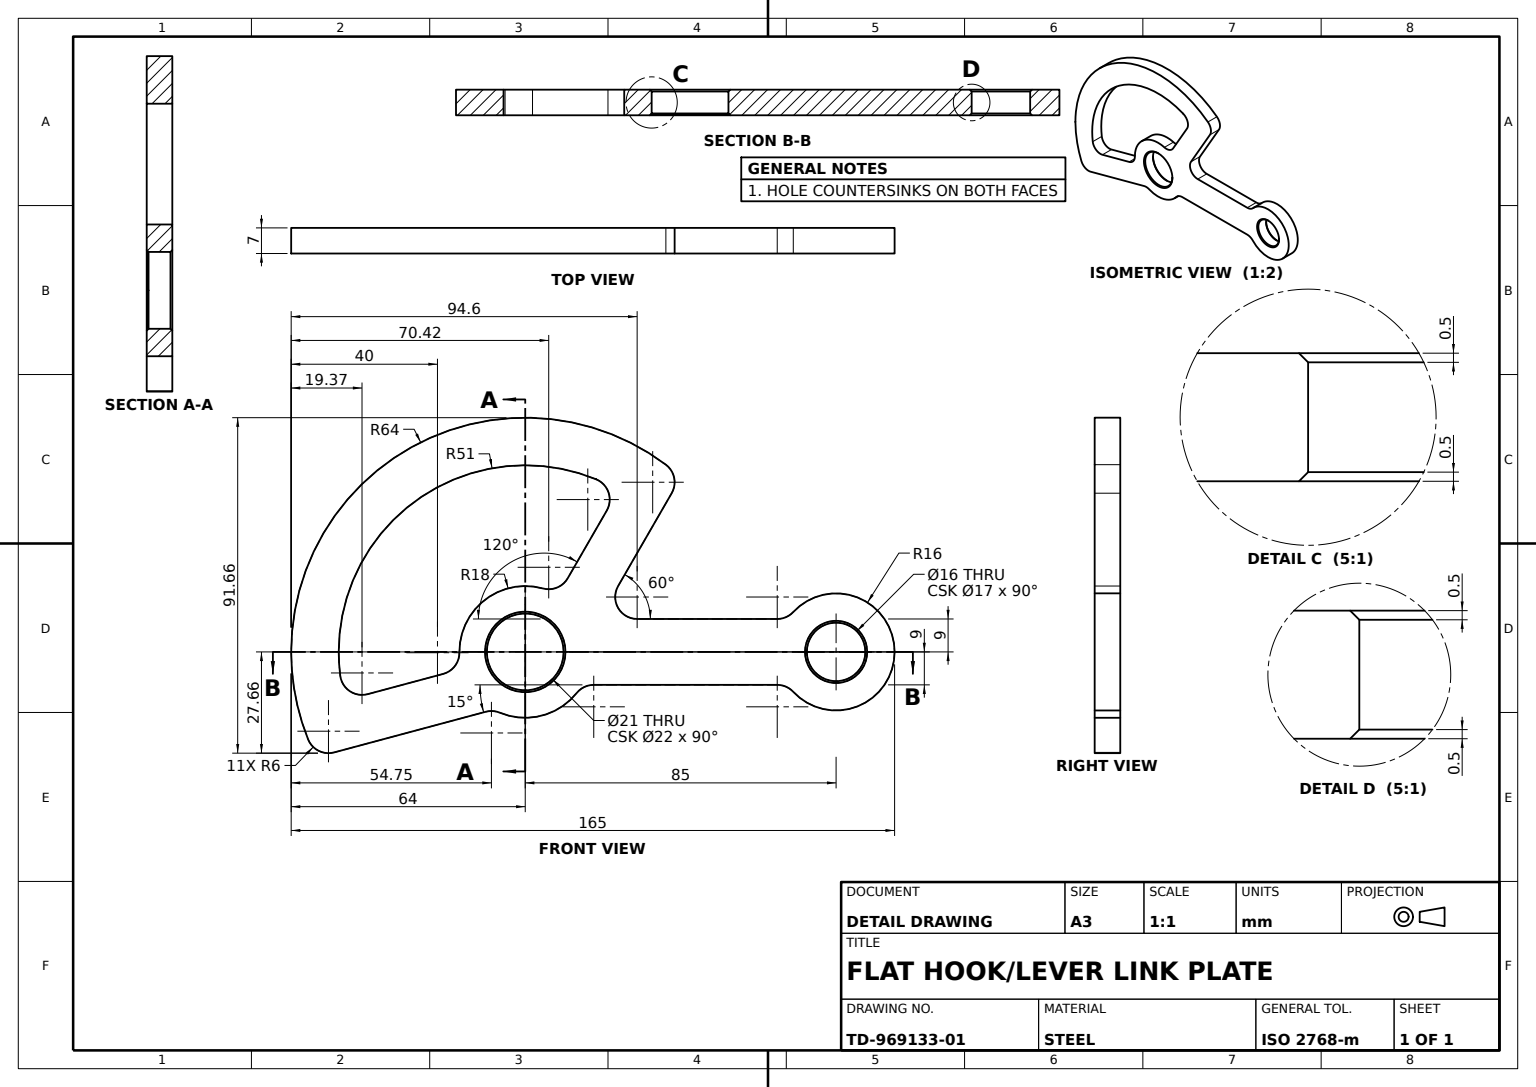
SolidWorks part; units mm, degrees
material "Plain Carbon Steel"
ref_plane "Front Plane" through (0, 0, 0) normal (0, 0, 1) x (1, 0, 0)
ref_plane "Top Plane" through (0, 0, 0) normal (0, 1, 0) x (1, 0, 0)
ref_plane "Right Plane" through (0, 0, 0) normal (1, 0, 0) x (0, 0, -1)
sketch "Opener Profile Sketch" plane through (0, 0, 0) normal (0, 0, 1) x (1, 0, 0)
  line L0 (0, 0) -> (85, 0) construction
  line L1 (20.2073, 9) -> (71.7712, 9)
  line L2 (15.5885, -9) -> (71.7712, -9)
  line L3 (9, 15.5885) -> (25.5, 44.1673)
  line L6 (0, 0) -> (-93.764, 0) construction
  line L8 (-8.661, -15.7793) -> (-57.1658, -28.7761)
  line L9 (20.2073, 9) -> (42.5912, 47.7702)
  line L10 (-17.3867, -4.6587) -> (-49.2622, -13.1998)
  circle A0 centre (85, 0) radius 8
  arc A1 (71.7712, -9) -> (71.7712, 9) centre (85, 0) ccw
  circle A2 centre (0, 0) radius 10.5
  arc A3 (-8.661, -15.7793) -> (15.5885, -9) centre (0, 0) ccw
  arc A5 (-57.1658, -28.7761) -> (42.5912, 47.7702) centre (0, 0) cw
  arc A6 (-49.2622, -13.1998) -> (25.5, 44.1673) centre (0, 0) cw
  arc A7 (9, 15.5885) -> (-17.3867, -4.6587) centre (0, 0) ccw
  point P18 (3.3646, -12.557)
  dimension "D2" = 32
  dimension "D3" = 16
  dimension "D4" = 21
  dimension "D5" = 36
  dimension "D8" = 13
  dimension "D9" = 13
  dimension "D11" = 64
  dimension "D12" = 51
  dimension "D14" = 49.2622
  dimension "D1" = 85
  dimension "D6" = 9
  dimension "D7" = 30
  dimension "D10" = 57.1658
  dimension "D13" = 42.5912
  dimension "D15" = 56.1828
extrude "Opener Plate 7mm" add sketch "Opener Profile Sketch" along normal mid plane 7
fillet "Edge Fillets R6" radius 6 11 edges at (20.2073, 9, 0) (-57.1658, -28.7761, 0) (42.5912, 47.7702, 0) (25.5, 44.1673, 0) (-49.2622, -13.1998, 0) (-17.3867, -4.6587, 0) (9, 15.5885, 0) (-8.661, -15.7793, 0) (15.5885, -9, 0) (71.7712, -9, 0) (71.7712, 9, 0)
chamfer "Edge Chamfers 0.5x45" distance 0.5 angle 45 4 edges at (93, 0, 3.5) (93, 0, -3.5) (10.5, 0, -3.5) (10.5, 0, 3.5)
